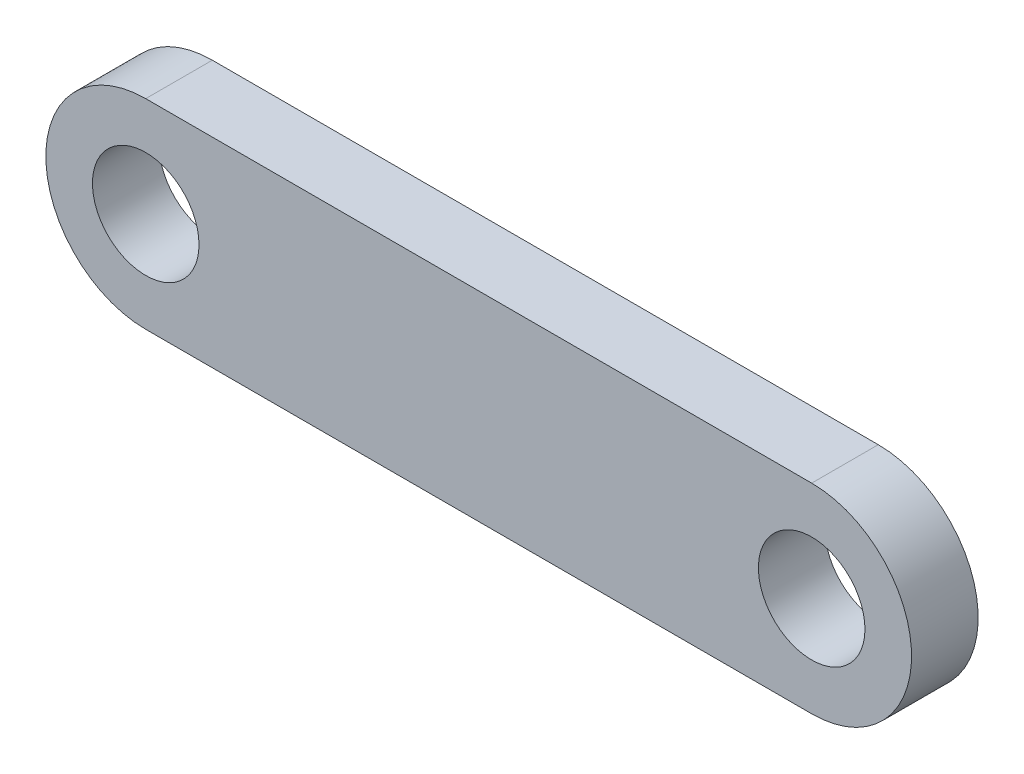
ISO-10303-21;
HEADER;
FILE_DESCRIPTION(('STEP AP214'),'2;1');
FILE_NAME('part.step','',(''),(''),'','','');
FILE_SCHEMA(('AUTOMOTIVE_DESIGN { 1 0 10303 214 1 1 1 1 }'));
ENDSEC;
DATA;
#1=APPLICATION_CONTEXT('core data for automotive mechanical design processes');
#2=APPLICATION_PROTOCOL_DEFINITION('international standard','automotive_design',2000,#1);
#3=PRODUCT_CONTEXT('',#1,'mechanical');
#4=PRODUCT('Part','Part','',(#3));
#5=PRODUCT_RELATED_PRODUCT_CATEGORY('part','',(#4));
#6=PRODUCT_DEFINITION_FORMATION('','',#4);
#7=PRODUCT_DEFINITION_CONTEXT('part definition',#1,'design');
#8=PRODUCT_DEFINITION('design','',#6,#7);
#9=PRODUCT_DEFINITION_SHAPE('','',#8);
#10=(LENGTH_UNIT() NAMED_UNIT(*) SI_UNIT(.MILLI.,.METRE.));
#11=(NAMED_UNIT(*) PLANE_ANGLE_UNIT() SI_UNIT($,.RADIAN.));
#12=(NAMED_UNIT(*) SI_UNIT($,.STERADIAN.) SOLID_ANGLE_UNIT());
#13=UNCERTAINTY_MEASURE_WITH_UNIT(LENGTH_MEASURE(1.E-05),#10,'distance_accuracy_value','');
#14=(GEOMETRIC_REPRESENTATION_CONTEXT(3) GLOBAL_UNCERTAINTY_ASSIGNED_CONTEXT((#13)) GLOBAL_UNIT_ASSIGNED_CONTEXT((#10,
#11,#12)) REPRESENTATION_CONTEXT('',''));
#15=CARTESIAN_POINT('',(0.,0.,0.));
#16=DIRECTION('',(0.,0.,1.));
#17=DIRECTION('',(1.,0.,0.));
#18=AXIS2_PLACEMENT_3D('',#15,#16,#17);
#19=CARTESIAN_POINT('',(25.,0.,2.5));
#20=DIRECTION('',(0.,0.,1.));
#21=DIRECTION('',(1.,0.,0.));
#22=AXIS2_PLACEMENT_3D('',#19,#20,#21);
#23=PLANE('',#22);
#24=CARTESIAN_POINT('',(-25.,0.,2.5));
#25=DIRECTION('',(0.,0.,1.));
#26=DIRECTION('',(1.,0.,0.));
#27=AXIS2_PLACEMENT_3D('',#24,#25,#26);
#28=CIRCLE('',#27,4.);
#29=CARTESIAN_POINT('',(-21.,0.,2.5));
#30=VERTEX_POINT('',#29);
#31=EDGE_CURVE('E107',#30,#30,#28,.T.);
#32=ORIENTED_EDGE('',*,*,#31,.F.);
#33=EDGE_LOOP('',(#32));
#34=FACE_BOUND('',#33,.T.);
#35=CARTESIAN_POINT('',(25.,0.,2.5));
#36=DIRECTION('',(0.,0.,1.));
#37=DIRECTION('',(1.,0.,0.));
#38=AXIS2_PLACEMENT_3D('',#35,#36,#37);
#39=CIRCLE('',#38,7.5);
#40=CARTESIAN_POINT('',(25.,-7.49999999999999,2.5));
#41=VERTEX_POINT('',#40);
#42=CARTESIAN_POINT('',(25.,7.50000000000001,2.5));
#43=VERTEX_POINT('',#42);
#44=EDGE_CURVE('E91',#41,#43,#39,.T.);
#45=ORIENTED_EDGE('',*,*,#44,.T.);
#46=DIRECTION('',(-1.,0.,0.));
#47=VECTOR('',#46,1.);
#48=CARTESIAN_POINT('',(25.,7.50000000000001,2.5));
#49=LINE('',#48,#47);
#50=CARTESIAN_POINT('',(-25.,7.5,2.5));
#51=VERTEX_POINT('',#50);
#52=EDGE_CURVE('E86',#43,#51,#49,.T.);
#53=ORIENTED_EDGE('',*,*,#52,.T.);
#54=CARTESIAN_POINT('',(-25.,0.,2.5));
#55=DIRECTION('',(0.,0.,1.));
#56=DIRECTION('',(1.,0.,0.));
#57=AXIS2_PLACEMENT_3D('',#54,#55,#56);
#58=CIRCLE('',#57,7.5);
#59=CARTESIAN_POINT('',(-25.,-7.5,2.5));
#60=VERTEX_POINT('',#59);
#61=EDGE_CURVE('E93',#51,#60,#58,.T.);
#62=ORIENTED_EDGE('',*,*,#61,.T.);
#63=DIRECTION('',(1.,0.,0.));
#64=VECTOR('',#63,1.);
#65=CARTESIAN_POINT('',(25.,-7.49999999999999,2.5));
#66=LINE('',#65,#64);
#67=EDGE_CURVE('E59',#60,#41,#66,.T.);
#68=ORIENTED_EDGE('',*,*,#67,.T.);
#69=EDGE_LOOP('',(#45,#53,#62,#68));
#70=FACE_BOUND('',#69,.T.);
#71=CARTESIAN_POINT('',(25.,0.,2.5));
#72=DIRECTION('',(0.,0.,1.));
#73=DIRECTION('',(1.,0.,0.));
#74=AXIS2_PLACEMENT_3D('',#71,#72,#73);
#75=CIRCLE('',#74,4.);
#76=CARTESIAN_POINT('',(29.,0.,2.5));
#77=VERTEX_POINT('',#76);
#78=EDGE_CURVE('E124',#77,#77,#75,.T.);
#79=ORIENTED_EDGE('',*,*,#78,.F.);
#80=EDGE_LOOP('',(#79));
#81=FACE_BOUND('',#80,.T.);
#82=ADVANCED_FACE('F41',(#34,#70,#81),#23,.T.);
#83=CARTESIAN_POINT('',(25.,0.,-2.5));
#84=DIRECTION('',(0.,0.,1.));
#85=DIRECTION('',(1.,0.,0.));
#86=AXIS2_PLACEMENT_3D('',#83,#84,#85);
#87=PLANE('',#86);
#88=CARTESIAN_POINT('',(25.,0.,-2.5));
#89=DIRECTION('',(0.,0.,1.));
#90=DIRECTION('',(1.,0.,0.));
#91=AXIS2_PLACEMENT_3D('',#88,#89,#90);
#92=CIRCLE('',#91,7.5);
#93=CARTESIAN_POINT('',(25.,-7.49999999999999,-2.5));
#94=VERTEX_POINT('',#93);
#95=CARTESIAN_POINT('',(25.,7.50000000000001,-2.5));
#96=VERTEX_POINT('',#95);
#97=EDGE_CURVE('E104',#94,#96,#92,.T.);
#98=ORIENTED_EDGE('',*,*,#97,.F.);
#99=DIRECTION('',(1.,0.,0.));
#100=VECTOR('',#99,1.);
#101=CARTESIAN_POINT('',(25.,-7.49999999999999,-2.5));
#102=LINE('',#101,#100);
#103=CARTESIAN_POINT('',(-25.,-7.5,-2.5));
#104=VERTEX_POINT('',#103);
#105=EDGE_CURVE('E82',#104,#94,#102,.T.);
#106=ORIENTED_EDGE('',*,*,#105,.F.);
#107=CARTESIAN_POINT('',(-25.,0.,-2.5));
#108=DIRECTION('',(0.,0.,1.));
#109=DIRECTION('',(1.,0.,0.));
#110=AXIS2_PLACEMENT_3D('',#107,#108,#109);
#111=CIRCLE('',#110,7.5);
#112=CARTESIAN_POINT('',(-25.,7.5,-2.5));
#113=VERTEX_POINT('',#112);
#114=EDGE_CURVE('E73',#113,#104,#111,.T.);
#115=ORIENTED_EDGE('',*,*,#114,.F.);
#116=DIRECTION('',(-1.,0.,0.));
#117=VECTOR('',#116,1.);
#118=CARTESIAN_POINT('',(25.,7.50000000000001,-2.5));
#119=LINE('',#118,#117);
#120=EDGE_CURVE('E100',#96,#113,#119,.T.);
#121=ORIENTED_EDGE('',*,*,#120,.F.);
#122=EDGE_LOOP('',(#98,#106,#115,#121));
#123=FACE_BOUND('',#122,.T.);
#124=CARTESIAN_POINT('',(-25.,0.,-2.5));
#125=DIRECTION('',(0.,0.,1.));
#126=DIRECTION('',(1.,0.,0.));
#127=AXIS2_PLACEMENT_3D('',#124,#125,#126);
#128=CIRCLE('',#127,4.);
#129=CARTESIAN_POINT('',(-21.,0.,-2.5));
#130=VERTEX_POINT('',#129);
#131=EDGE_CURVE('E118',#130,#130,#128,.T.);
#132=ORIENTED_EDGE('',*,*,#131,.T.);
#133=EDGE_LOOP('',(#132));
#134=FACE_BOUND('',#133,.T.);
#135=CARTESIAN_POINT('',(25.,0.,-2.5));
#136=DIRECTION('',(0.,0.,1.));
#137=DIRECTION('',(1.,0.,0.));
#138=AXIS2_PLACEMENT_3D('',#135,#136,#137);
#139=CIRCLE('',#138,4.);
#140=CARTESIAN_POINT('',(29.,0.,-2.5));
#141=VERTEX_POINT('',#140);
#142=EDGE_CURVE('E127',#141,#141,#139,.T.);
#143=ORIENTED_EDGE('',*,*,#142,.T.);
#144=EDGE_LOOP('',(#143));
#145=FACE_BOUND('',#144,.T.);
#146=ADVANCED_FACE('F117',(#123,#134,#145),#87,.F.);
#147=CARTESIAN_POINT('',(25.,0.,2.5));
#148=DIRECTION('',(0.,0.,-1.));
#149=DIRECTION('',(-1.,0.,0.));
#150=AXIS2_PLACEMENT_3D('',#147,#148,#149);
#151=CYLINDRICAL_SURFACE('',#150,7.5);
#152=ORIENTED_EDGE('',*,*,#97,.T.);
#153=DIRECTION('',(0.,0.,-1.));
#154=VECTOR('',#153,1.);
#155=CARTESIAN_POINT('',(25.,7.50000000000001,2.5));
#156=LINE('',#155,#154);
#157=EDGE_CURVE('E11',#43,#96,#156,.T.);
#158=ORIENTED_EDGE('',*,*,#157,.F.);
#159=ORIENTED_EDGE('',*,*,#44,.F.);
#160=DIRECTION('',(0.,0.,-1.));
#161=VECTOR('',#160,1.);
#162=CARTESIAN_POINT('',(25.,-7.49999999999999,2.5));
#163=LINE('',#162,#161);
#164=EDGE_CURVE('E101',#41,#94,#163,.T.);
#165=ORIENTED_EDGE('',*,*,#164,.T.);
#166=EDGE_LOOP('',(#152,#158,#159,#165));
#167=FACE_BOUND('',#166,.T.);
#168=ADVANCED_FACE('F43',(#167),#151,.T.);
#169=CARTESIAN_POINT('',(25.,7.50000000000001,2.5));
#170=DIRECTION('',(0.,-1.,0.));
#171=DIRECTION('',(1.,0.,0.));
#172=AXIS2_PLACEMENT_3D('',#169,#170,#171);
#173=PLANE('',#172);
#174=ORIENTED_EDGE('',*,*,#120,.T.);
#175=DIRECTION('',(0.,0.,-1.));
#176=VECTOR('',#175,1.);
#177=CARTESIAN_POINT('',(-25.,7.5,2.5));
#178=LINE('',#177,#176);
#179=EDGE_CURVE('E49',#51,#113,#178,.T.);
#180=ORIENTED_EDGE('',*,*,#179,.F.);
#181=ORIENTED_EDGE('',*,*,#52,.F.);
#182=ORIENTED_EDGE('',*,*,#157,.T.);
#183=EDGE_LOOP('',(#174,#180,#181,#182));
#184=FACE_BOUND('',#183,.T.);
#185=ADVANCED_FACE('F96',(#184),#173,.F.);
#186=CARTESIAN_POINT('',(-25.,0.,2.5));
#187=DIRECTION('',(0.,0.,-1.));
#188=DIRECTION('',(-1.,0.,0.));
#189=AXIS2_PLACEMENT_3D('',#186,#187,#188);
#190=CYLINDRICAL_SURFACE('',#189,7.5);
#191=ORIENTED_EDGE('',*,*,#114,.T.);
#192=DIRECTION('',(0.,0.,-1.));
#193=VECTOR('',#192,1.);
#194=CARTESIAN_POINT('',(-25.,-7.5,2.5));
#195=LINE('',#194,#193);
#196=EDGE_CURVE('E98',#60,#104,#195,.T.);
#197=ORIENTED_EDGE('',*,*,#196,.F.);
#198=ORIENTED_EDGE('',*,*,#61,.F.);
#199=ORIENTED_EDGE('',*,*,#179,.T.);
#200=EDGE_LOOP('',(#191,#197,#198,#199));
#201=FACE_BOUND('',#200,.T.);
#202=ADVANCED_FACE('F97',(#201),#190,.T.);
#203=CARTESIAN_POINT('',(25.,-7.49999999999999,2.5));
#204=DIRECTION('',(0.,1.,0.));
#205=DIRECTION('',(-1.,0.,0.));
#206=AXIS2_PLACEMENT_3D('',#203,#204,#205);
#207=PLANE('',#206);
#208=ORIENTED_EDGE('',*,*,#105,.T.);
#209=ORIENTED_EDGE('',*,*,#164,.F.);
#210=ORIENTED_EDGE('',*,*,#67,.F.);
#211=ORIENTED_EDGE('',*,*,#196,.T.);
#212=EDGE_LOOP('',(#208,#209,#210,#211));
#213=FACE_BOUND('',#212,.T.);
#214=ADVANCED_FACE('F114',(#213),#207,.F.);
#215=CARTESIAN_POINT('',(-25.,0.,2.5));
#216=DIRECTION('',(0.,0.,-1.));
#217=DIRECTION('',(-1.,0.,0.));
#218=AXIS2_PLACEMENT_3D('',#215,#216,#217);
#219=CYLINDRICAL_SURFACE('',#218,4.);
#220=ORIENTED_EDGE('',*,*,#31,.T.);
#221=EDGE_LOOP('',(#220));
#222=FACE_BOUND('',#221,.T.);
#223=ORIENTED_EDGE('',*,*,#131,.F.);
#224=EDGE_LOOP('',(#223));
#225=FACE_BOUND('',#224,.T.);
#226=ADVANCED_FACE('F141',(#222,#225),#219,.F.);
#227=CARTESIAN_POINT('',(25.,0.,2.5));
#228=DIRECTION('',(0.,0.,-1.));
#229=DIRECTION('',(-1.,0.,0.));
#230=AXIS2_PLACEMENT_3D('',#227,#228,#229);
#231=CYLINDRICAL_SURFACE('',#230,4.);
#232=ORIENTED_EDGE('',*,*,#78,.T.);
#233=EDGE_LOOP('',(#232));
#234=FACE_BOUND('',#233,.T.);
#235=ORIENTED_EDGE('',*,*,#142,.F.);
#236=EDGE_LOOP('',(#235));
#237=FACE_BOUND('',#236,.T.);
#238=ADVANCED_FACE('F135',(#234,#237),#231,.F.);
#239=CLOSED_SHELL('',(#82,#146,#168,#185,#202,#214,#226,#238));
#240=MANIFOLD_SOLID_BREP('B2',#239);
#241=ADVANCED_BREP_SHAPE_REPRESENTATION('',(#18,#240),#14);
#242=SHAPE_DEFINITION_REPRESENTATION(#9,#241);
ENDSEC;
END-ISO-10303-21;
